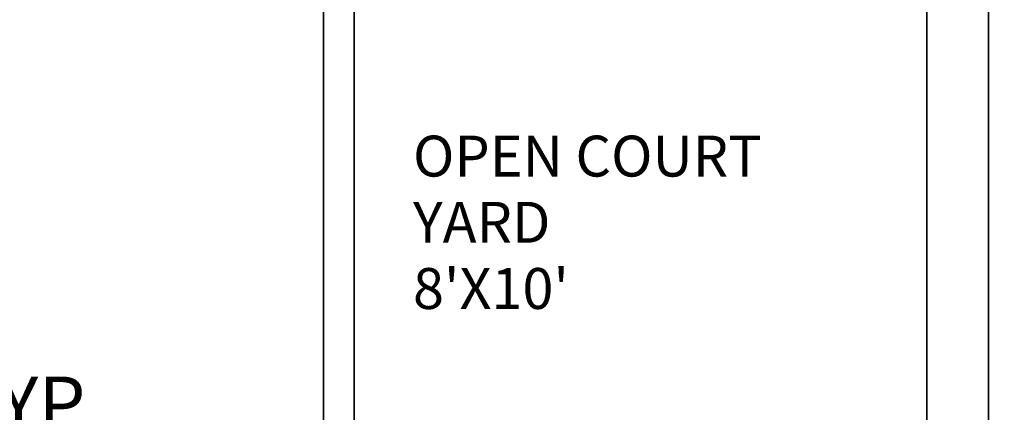
# Model space of a CAD drawing. Units: inches. Extents: x 125 to 976, y 231 to 853.
# Tile 9 of 16: x 324 to 468, y 555 to 613. Entities that reach past the tile are written whole.
import ezdxf

# ---------------------------------------------------------------- set-up
doc = ezdxf.new("R2010")
doc.units = ezdxf.units.IN
doc.header["$MEASUREMENT"] = 0
for name, color, linetype, lineweight in [('A-ANNO-DIMS', 2, 'Continuous', 18), ('A-AREA-IDEN', 7, 'Continuous', 18), ('A-WALL', 7, 'Continuous', 35)]:
    doc.layers.add(name, color=color, linetype=linetype, lineweight=lineweight)
doc.styles.get("Standard").update_dxf_attribs({"font": 'italic8.shx'})
doc.dimstyles.get("Standard").update_dxf_attribs({"dimtxt": 8, "dimasz": 0.18, "dimexe": 0.18, "dimexo": 0.0625, "dimgap": 0.09, "dimtad": 0, "dimtih": 1, "dimtoh": 1, "dimdec": 4, "dimzin": 0, "dimdsep": 46, "dimlunit": 3, "dimtxsty": 'Standard', "dimcen": 0.09, "dimclrt": 4, "dimadec": 0, "dimazin": 0, "dimtfac": 1, "dimtdec": 4, "dimtofl": 0, "dimtmove": 0, "dimatfit": 3, "dimfxl": 1, "dimtolj": 1, "dimtzin": 0, "dimarcsym": 0})

# ---------------------------------------------------------------- blocks, each defined once
blk = doc.blocks.new('*D46')
at = {"layer": 'A-ANNO-DIMS', "color": 0, "lineweight": -2, "transparency": 16777216}
for p, q in [((274.61, 567.59), (278.15, 567.59)), ((277.97, 567.41), (277.97, 561.05)), ((277.97, 544.97), (277.97, 551.34)), ((274.61, 544.79), (278.15, 544.79))]:
    blk.add_line(p, q, dxfattribs=at)
at = {"layer": 'A-ANNO-DIMS', "color": 0, "transparency": 16777216}
for points in [[(277.94, 567.41), (278, 567.41), (277.97, 567.59)], [(277.94, 544.97), (278, 544.97), (277.97, 544.79)]]:
    blk.add_solid(points, dxfattribs=at)
at = {"layer": 'Defpoints', "color": 0, "transparency": 16777216}
for p in [(274.55, 567.59), (277.97, 567.59), (274.55, 544.79)]:
    blk.add_point(p, dxfattribs=at)
at = {"layer": 'A-ANNO-DIMS', "color": 4, "transparency": 16777216, "insert": (277.97, 556.19), "char_height": 8, "attachment_point": 5}
blk.add_mtext('\\A1;DINING SET 1\'-11" TYP.', dxfattribs=at)
blk = doc.blocks.new('*D64')
at = {"layer": 'A-ANNO-DIMS', "color": 0, "lineweight": -2, "transparency": 16777216}
for p, q in [((465.64, 658.83), (494.46, 658.83)), ((494.28, 658.65), (494.28, 561.16)), ((494.28, 451.31), (494.28, 548.79)), ((465.64, 451.13), (494.46, 451.13))]:
    blk.add_line(p, q, dxfattribs=at)
at = {"layer": 'A-ANNO-DIMS', "color": 0, "transparency": 16777216}
for points in [[(494.25, 658.65), (494.31, 658.65), (494.28, 658.83)], [(494.25, 451.31), (494.31, 451.31), (494.28, 451.13)]]:
    blk.add_solid(points, dxfattribs=at)
at = {"layer": 'Defpoints', "color": 0, "transparency": 16777216}
for p in [(465.58, 658.83), (494.28, 658.83), (465.58, 451.13)]:
    blk.add_point(p, dxfattribs=at)
at = {"layer": 'A-ANNO-DIMS', "color": 4, "transparency": 16777216, "insert": (494.28, 554.98), "char_height": 8, "attachment_point": 5}
blk.add_mtext('\\A1;17\'-3 1/2"', dxfattribs=at)

msp = doc.modelspace()

# ---------------------------------------------------------------- linework, layer by layer
at = {"layer": 'A-WALL'}
for p, q in [((368.0792, 614.10475), (368.0792, 503.10475)), ((372.5792, 614.10475), (372.5792, 503.10475)), ((456.5792, 503.10475), (456.5792, 614.10475))]:
    msp.add_line(p, q, dxfattribs=at)
msp.add_lwpolyline([(177.5792, 272.10475), (465.5792, 272.10475), (465.5792, 812.10475), (177.5792, 812.10475)], close=True, dxfattribs=at)

# ---------------------------------------------------------------- texts
at = {"layer": 'A-AREA-IDEN'}
for s, p in [('OPEN COURT', (381.1988, 589.5314)), ('YARD', (381.1988, 579.81711)), ("8'X10'", (381.1988, 570.10282))]:
    msp.add_text(s, height=6, dxfattribs=at).set_placement(p)

# ---------------------------------------------------------------- dimensions: what is measured, and where the dimension line sits
at = {"layer": 'A-ANNO-DIMS'}
dim = msp.add_linear_dim(base=(494.2792, 658.82838), p1=(465.5792, 451.12515), p2=(465.5792, 658.82838), angle=90, dimstyle='Standard', override={"dimdec": 1, "dimlfac": 1, "dimrnd": 0, "dimzin": 1, "dimdsep": 46, "dimlunit": 4, "dimfrac": 2}, dxfattribs=at)
dim.commit()
dim.dimension.update_dxf_attribs({"geometry": '*D64', "text_midpoint": (494.2792, 554.97677)})
dim = msp.add_linear_dim(base=(277.96826, 567.59411), p1=(274.54835, 544.79468), p2=(274.54835, 567.59411), angle=90, text='DINING SET <> TYP.', dimstyle='Standard', override={"dimdec": 1, "dimlfac": 1, "dimrnd": 0, "dimzin": 1, "dimdsep": 46, "dimlunit": 4, "dimfrac": 2}, dxfattribs=at)
dim.commit()
dim.dimension.update_dxf_attribs({"geometry": '*D46', "text_midpoint": (277.96826, 556.1944)})

doc.saveas('drawing.dxf')
